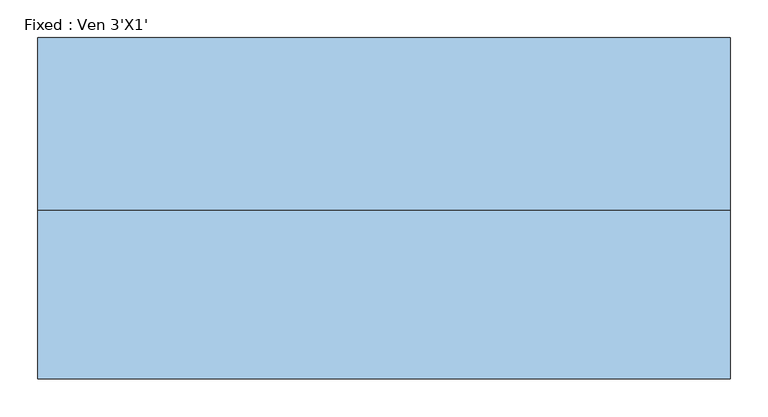
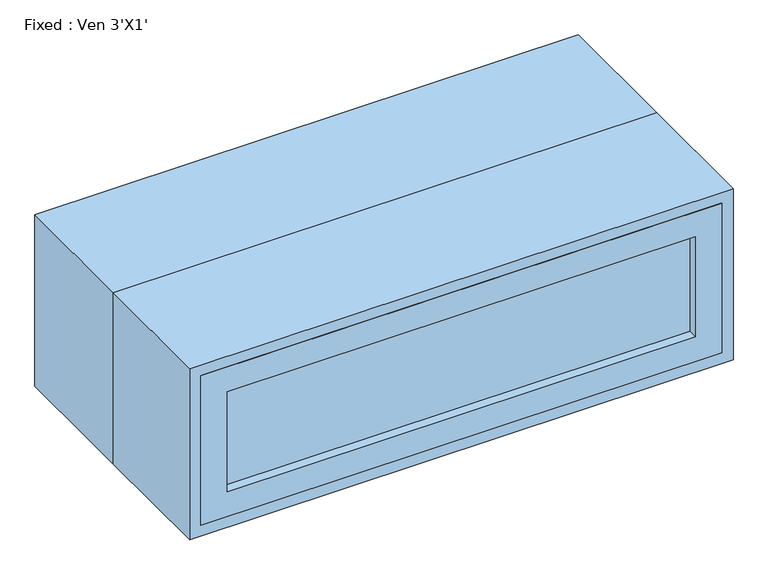
"""IFC4 building model written with IfcOpenShell, lengths in millimetres: window geometry, Fixed : Ven 3'X1'."""

from ifc_helpers import new_model, si_unit, frame, origin, place, context, project, spatial, polyline, outline, extrude, source, transform, mapped, element, save


def fixed_ven_3_x1_1ea7015b(model_context):
    return source(origin(), model_context, "Body", "SweptSolid", [
        extrude(outline(polyline([(355.6, -320.675), (-431.8, -320.675), (-431.8, -307.975), (355.6, -307.975), (355.6, -320.675)])), frame((0.0, 0.0, 2197.1), z_axis=(0.0, 0.0, 1.0), x_axis=(1.0, 0.0, 0.0)), (0.0, 0.0, 1.0), 177.8),
        extrude(outline(polyline([(2419.35, -476.25), (2152.65, -476.25), (2152.65, 400.05), (2419.35, 400.05), (2419.35, -476.25)]), holes=[polyline([(2374.9, -431.8), (2374.9, 355.6), (2197.1, 355.6), (2197.1, -431.8), (2374.9, -431.8)])]), frame((0.0, -336.55, 0.0), z_axis=(0.0, 1.0, 0.0), x_axis=(0.0, 0.0, 1.0)), (0.0, 0.0, 1.0), 44.45),
        extrude(outline(polyline([(2438.4, -495.3), (2133.6, -495.3), (2133.6, 419.1), (2438.4, 419.1), (2438.4, -495.3)]), holes=[polyline([(2406.65, -463.55), (2406.65, 387.35), (2165.35, 387.35), (2165.35, -463.55), (2406.65, -463.55)])]), frame((0.0, -336.55, 0.0), z_axis=(0.0, 1.0, 0.0), x_axis=(0.0, 0.0, 1.0)), (0.0, 0.0, 1.0), 222.25),
        extrude(outline(polyline([(2438.4, 419.1), (2438.4, -495.3), (2133.6, -495.3), (2133.6, 419.1), (2438.4, 419.1)]), holes=[polyline([(2419.35, 400.05), (2152.65, 400.05), (2152.65, -476.25), (2419.35, -476.25), (2419.35, 400.05)])]), frame((0.0, -336.55, 0.0), z_axis=(0.0, 1.0, 0.0), x_axis=(0.0, 0.0, 1.0)), (0.0, 0.0, 1.0), 450.85),
    ])


if __name__ == "__main__":
    model = new_model("IFC4")
    model_context = context("Model", 3, world=origin())
    ifc_project = project(units=[si_unit("LENGTHUNIT", "METRE", prefix="MILLI")], contexts=[model_context])
    site = spatial("IfcSite", under=ifc_project)
    building = spatial("IfcBuilding", under=site)
    placement = place(None, origin())
    fixed_ven_3_x1_shape = fixed_ven_3_x1_1ea7015b(model_context)
    element("IfcWindow", 1, ObjectType="Fixed : Ven 3'X1'", at=placement, inside=building, context=model_context, shape_type="MappedRepresentation", body=[
        mapped(fixed_ven_3_x1_shape, transform((0.0, 0.0, 0.0), x_axis=(1.0, 0.0, 0.0), y_axis=(0.0, 1.0, 0.0), z_axis=(0.0, 0.0, 1.0))),
    ])
    save(model, "model.ifc")

# Revit data of these elements
# Type "Fixed : Ven 3'X1'"
#   Type Mark = "32"
#   Construction Type Id = "GSP4R"
#   Assembly Code = "B2020100"
#   Analytic Construction = "1/8 in Pilkington single glazing"
#   Rough Width = 3' - 0"
#   Rough Height = 1' - 0"
#   Visual Light Transmittance = 0.9
#   Solar Heat Gain Coefficient = 0.78
#   Heat Transfer Coefficient (U) = 0.6496 BTU/(h·ft²·°F)
#   Height = 1' - 0"
#   Default Sill Height = 7' - 0"
#   Width = 3' - 0"
#   Window Inset = 1' - 4"
#   Define Thermal Properties by = 1
#   Glass Pane Material = Glass
#   Sash Material = Sash
#   Wall Closure = (empty or 0)
# Element 1 (IfcWindow, "Fixed : Ven 3'X1'")
#   Materials on its faces: "Sash", "Glass"
# Materials
#   "Glass": class "Glass", colour RGB 0 128 192, transparency 0.75, Description = "Soda Lime Glass", Cost = 0
#   "Sash": class "Wood", colour RGB 224 178 126, transparency 0, Cost = 0
